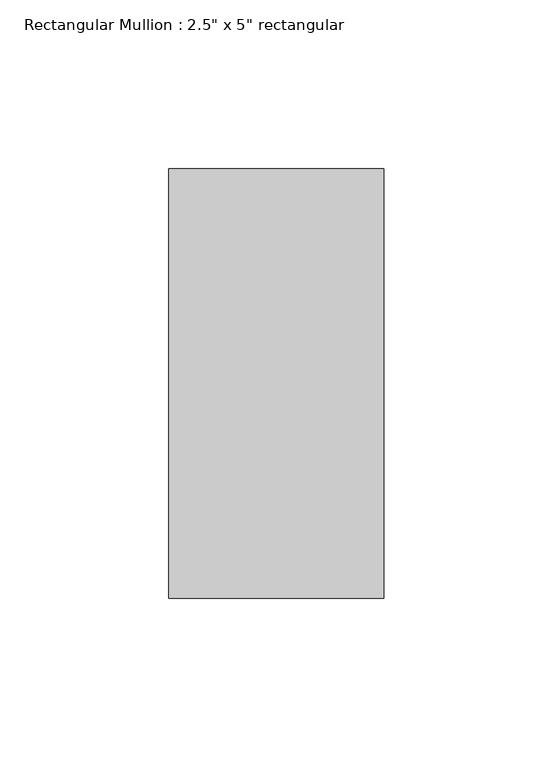
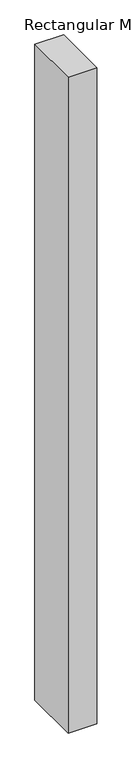
"""IFC4 building model written with IfcOpenShell, lengths in millimetres: member geometry."""

from ifc_helpers import new_model, si_unit, frame, origin, place, context, project, spatial, polyline, outline, extrude, source, transform, mapped, element, save


def member_4b34273c(model_context):
    return source(origin(), model_context, "Body", "SweptSolid", [
        extrude(outline(polyline([(31.75, 63.5), (31.75, -63.5), (-31.75, -63.5), (-31.75, 63.5), (31.75, 63.5)])), frame((0.0, 0.0, -1533.247479), z_axis=(0.0, 0.0, 1.0), x_axis=(1.0, 0.0, 0.0)), (0.0, 0.0, 1.0), 1533.247479),
    ])


if __name__ == "__main__":
    model = new_model("IFC4")
    model_context = context("Model", 3, world=origin())
    ifc_project = project(units=[si_unit("LENGTHUNIT", "METRE", prefix="MILLI")], contexts=[model_context])
    site = spatial("IfcSite", under=ifc_project)
    building = spatial("IfcBuilding", under=site)
    placement = place(None, origin())
    member_shape = member_4b34273c(model_context)
    element("IfcMember", 1, ObjectType="Rectangular Mullion : 2.5\" x 5\" rectangular", at=placement, inside=building, context=model_context, shape_type="MappedRepresentation", body=[
        mapped(member_shape, transform((0.0, 0.0, 0.0), x_axis=(1.0, 0.0, 0.0), y_axis=(0.0, 1.0, 0.0), z_axis=(0.0, 0.0, 1.0))),
    ])
    save(model, "model.ifc")

# Revit data of these elements
# Type "Rectangular Mullion : 2.5\" x 5\" rectangular"
#   built-in parameter 1007304 = 0.416667 (stored number, unit not read)
#   built-in parameter 1007301 = 0.104167 (stored number, unit not read)
#   built-in parameter 1007300 = 0.104167 (stored number, unit not read)
# Element 1 (IfcMember, "Rectangular Mullion : 2.5\" x 5\" rectangular")
#   Materials on its faces: "Aluminum"
# Materials
#   "Aluminum": class "Metal", colour RGB 247 247 247, transparency 0, Description = "Aluminum 6061", Cost = 0
